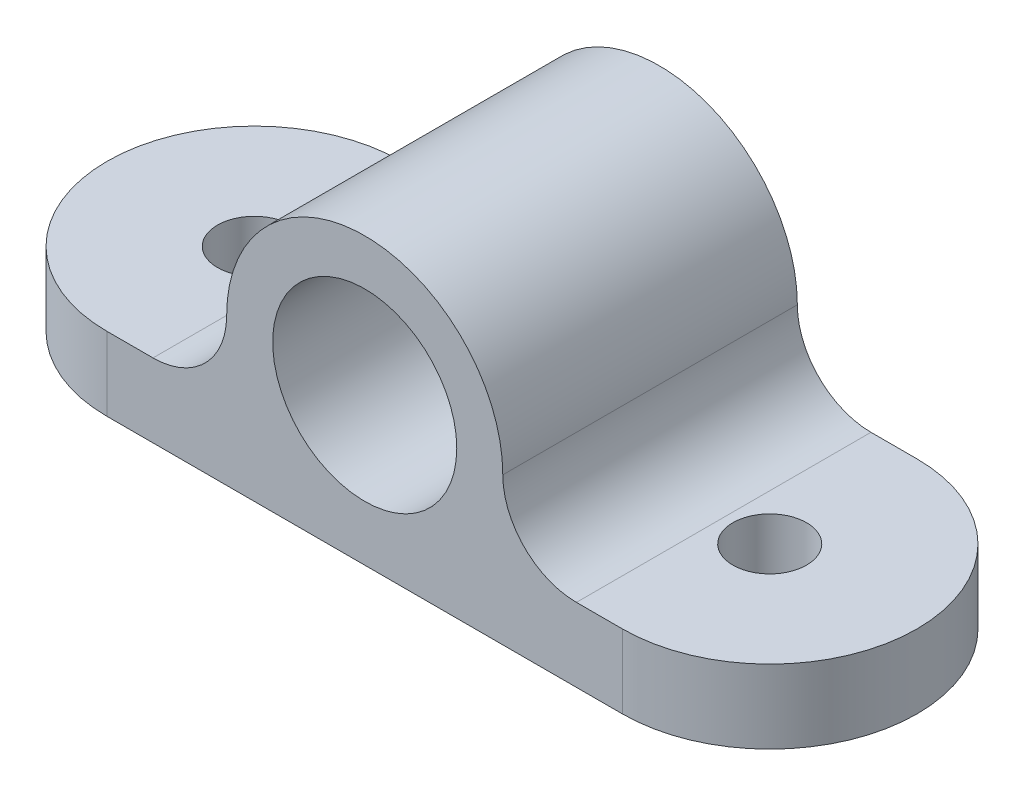
ISO-10303-21;
HEADER;
FILE_DESCRIPTION(('STEP AP214'),'2;1');
FILE_NAME('part.step','',(''),(''),'','','');
FILE_SCHEMA(('AUTOMOTIVE_DESIGN { 1 0 10303 214 1 1 1 1 }'));
ENDSEC;
DATA;
#1=APPLICATION_CONTEXT('core data for automotive mechanical design processes');
#2=APPLICATION_PROTOCOL_DEFINITION('international standard','automotive_design',2000,#1);
#3=PRODUCT_CONTEXT('',#1,'mechanical');
#4=PRODUCT('Part','Part','',(#3));
#5=PRODUCT_RELATED_PRODUCT_CATEGORY('part','',(#4));
#6=PRODUCT_DEFINITION_FORMATION('','',#4);
#7=PRODUCT_DEFINITION_CONTEXT('part definition',#1,'design');
#8=PRODUCT_DEFINITION('design','',#6,#7);
#9=PRODUCT_DEFINITION_SHAPE('','',#8);
#10=(LENGTH_UNIT() NAMED_UNIT(*) SI_UNIT(.MILLI.,.METRE.));
#11=(NAMED_UNIT(*) PLANE_ANGLE_UNIT() SI_UNIT($,.RADIAN.));
#12=(NAMED_UNIT(*) SI_UNIT($,.STERADIAN.) SOLID_ANGLE_UNIT());
#13=UNCERTAINTY_MEASURE_WITH_UNIT(LENGTH_MEASURE(1.E-05),#10,'distance_accuracy_value','');
#14=(GEOMETRIC_REPRESENTATION_CONTEXT(3) GLOBAL_UNCERTAINTY_ASSIGNED_CONTEXT((#13)) GLOBAL_UNIT_ASSIGNED_CONTEXT((#10,
#11,#12)) REPRESENTATION_CONTEXT('',''));
#15=CARTESIAN_POINT('',(0.,0.,0.));
#16=DIRECTION('',(0.,0.,1.));
#17=DIRECTION('',(1.,0.,0.));
#18=AXIS2_PLACEMENT_3D('',#15,#16,#17);
#19=CARTESIAN_POINT('',(-70.,0.,40.));
#20=DIRECTION('',(0.,-1.,0.));
#21=DIRECTION('',(0.,0.,-1.));
#22=AXIS2_PLACEMENT_3D('',#19,#20,#21);
#23=CYLINDRICAL_SURFACE('',#22,40.);
#24=DIRECTION('',(0.,-1.,0.));
#25=VECTOR('',#24,1.);
#26=CARTESIAN_POINT('',(-70.,40.,0.));
#27=LINE('',#26,#25);
#28=CARTESIAN_POINT('',(-70.,0.,0.));
#29=VERTEX_POINT('',#28);
#30=CARTESIAN_POINT('',(-70.,20.,0.));
#31=VERTEX_POINT('',#30);
#32=EDGE_CURVE('E154',#29,#31,#27,.F.);
#33=ORIENTED_EDGE('',*,*,#32,.F.);
#34=CARTESIAN_POINT('',(-70.,0.,40.));
#35=DIRECTION('',(0.,1.,0.));
#36=DIRECTION('',(0.,0.,1.));
#37=AXIS2_PLACEMENT_3D('',#34,#35,#36);
#38=CIRCLE('',#37,40.);
#39=CARTESIAN_POINT('',(-70.,0.,80.));
#40=VERTEX_POINT('',#39);
#41=EDGE_CURVE('E49',#40,#29,#38,.F.);
#42=ORIENTED_EDGE('',*,*,#41,.F.);
#43=DIRECTION('',(0.,1.,0.));
#44=VECTOR('',#43,1.);
#45=CARTESIAN_POINT('',(-70.,0.,80.));
#46=LINE('',#45,#44);
#47=CARTESIAN_POINT('',(-70.,20.,80.));
#48=VERTEX_POINT('',#47);
#49=EDGE_CURVE('E158',#48,#40,#46,.F.);
#50=ORIENTED_EDGE('',*,*,#49,.F.);
#51=CARTESIAN_POINT('',(-70.,20.,40.));
#52=DIRECTION('',(0.,-1.,0.));
#53=DIRECTION('',(0.,0.,-1.));
#54=AXIS2_PLACEMENT_3D('',#51,#52,#53);
#55=CIRCLE('',#54,40.);
#56=EDGE_CURVE('E11',#31,#48,#55,.F.);
#57=ORIENTED_EDGE('',*,*,#56,.F.);
#58=EDGE_LOOP('',(#33,#42,#50,#57));
#59=FACE_BOUND('',#58,.T.);
#60=ADVANCED_FACE('F41',(#59),#23,.T.);
#61=CARTESIAN_POINT('',(70.,0.,40.));
#62=DIRECTION('',(0.,1.,0.));
#63=DIRECTION('',(0.,0.,1.));
#64=AXIS2_PLACEMENT_3D('',#61,#62,#63);
#65=CYLINDRICAL_SURFACE('',#64,40.);
#66=DIRECTION('',(0.,-1.,0.));
#67=VECTOR('',#66,1.);
#68=CARTESIAN_POINT('',(70.,0.,80.));
#69=LINE('',#68,#67);
#70=CARTESIAN_POINT('',(70.,0.,80.));
#71=VERTEX_POINT('',#70);
#72=CARTESIAN_POINT('',(70.,20.,80.));
#73=VERTEX_POINT('',#72);
#74=EDGE_CURVE('E145',#71,#73,#69,.F.);
#75=ORIENTED_EDGE('',*,*,#74,.F.);
#76=CARTESIAN_POINT('',(70.,0.,40.));
#77=DIRECTION('',(0.,1.,0.));
#78=DIRECTION('',(0.,0.,1.));
#79=AXIS2_PLACEMENT_3D('',#76,#77,#78);
#80=CIRCLE('',#79,40.);
#81=CARTESIAN_POINT('',(70.,0.,0.));
#82=VERTEX_POINT('',#81);
#83=EDGE_CURVE('E147',#82,#71,#80,.F.);
#84=ORIENTED_EDGE('',*,*,#83,.F.);
#85=DIRECTION('',(0.,1.,0.));
#86=VECTOR('',#85,1.);
#87=CARTESIAN_POINT('',(70.,40.,0.));
#88=LINE('',#87,#86);
#89=CARTESIAN_POINT('',(70.,20.,0.));
#90=VERTEX_POINT('',#89);
#91=EDGE_CURVE('E150',#90,#82,#88,.F.);
#92=ORIENTED_EDGE('',*,*,#91,.F.);
#93=CARTESIAN_POINT('',(70.,20.,40.));
#94=DIRECTION('',(0.,-1.,0.));
#95=DIRECTION('',(0.,0.,-1.));
#96=AXIS2_PLACEMENT_3D('',#93,#94,#95);
#97=CIRCLE('',#96,40.);
#98=EDGE_CURVE('E153',#73,#90,#97,.F.);
#99=ORIENTED_EDGE('',*,*,#98,.F.);
#100=EDGE_LOOP('',(#75,#84,#92,#99));
#101=FACE_BOUND('',#100,.T.);
#102=ADVANCED_FACE('F213',(#101),#65,.T.);
#103=CARTESIAN_POINT('',(0.,40.,80.));
#104=DIRECTION('',(0.,0.,1.));
#105=DIRECTION('',(1.,0.,0.));
#106=AXIS2_PLACEMENT_3D('',#103,#104,#105);
#107=PLANE('',#106);
#108=DIRECTION('',(-1.,0.,0.));
#109=VECTOR('',#108,1.);
#110=CARTESIAN_POINT('',(-37.5,20.,80.));
#111=LINE('',#110,#109);
#112=CARTESIAN_POINT('',(-57.5,20.,80.));
#113=VERTEX_POINT('',#112);
#114=EDGE_CURVE('E116',#113,#48,#111,.T.);
#115=ORIENTED_EDGE('',*,*,#114,.T.);
#116=ORIENTED_EDGE('',*,*,#49,.T.);
#117=DIRECTION('',(1.,0.,0.));
#118=VECTOR('',#117,1.);
#119=CARTESIAN_POINT('',(-110.,0.,80.));
#120=LINE('',#119,#118);
#121=EDGE_CURVE('E167',#40,#71,#120,.T.);
#122=ORIENTED_EDGE('',*,*,#121,.T.);
#123=ORIENTED_EDGE('',*,*,#74,.T.);
#124=DIRECTION('',(-1.,0.,0.));
#125=VECTOR('',#124,1.);
#126=CARTESIAN_POINT('',(110.,20.,80.));
#127=LINE('',#126,#125);
#128=CARTESIAN_POINT('',(57.5,20.,80.));
#129=VERTEX_POINT('',#128);
#130=EDGE_CURVE('E178',#73,#129,#127,.T.);
#131=ORIENTED_EDGE('',*,*,#130,.T.);
#132=CARTESIAN_POINT('',(57.5,40.,80.));
#133=DIRECTION('',(0.,0.,1.));
#134=DIRECTION('',(1.,0.,0.));
#135=AXIS2_PLACEMENT_3D('',#132,#133,#134);
#136=CIRCLE('',#135,20.);
#137=CARTESIAN_POINT('',(37.5,40.,80.));
#138=VERTEX_POINT('',#137);
#139=EDGE_CURVE('E115',#129,#138,#136,.F.);
#140=ORIENTED_EDGE('',*,*,#139,.T.);
#141=CARTESIAN_POINT('',(0.,40.,80.));
#142=DIRECTION('',(0.,0.,1.));
#143=DIRECTION('',(1.,0.,0.));
#144=AXIS2_PLACEMENT_3D('',#141,#142,#143);
#145=CIRCLE('',#144,37.5);
#146=CARTESIAN_POINT('',(-37.5,40.,80.));
#147=VERTEX_POINT('',#146);
#148=EDGE_CURVE('E102',#138,#147,#145,.T.);
#149=ORIENTED_EDGE('',*,*,#148,.T.);
#150=CARTESIAN_POINT('',(-57.5,40.,80.));
#151=DIRECTION('',(0.,0.,1.));
#152=DIRECTION('',(1.,0.,0.));
#153=AXIS2_PLACEMENT_3D('',#150,#151,#152);
#154=CIRCLE('',#153,20.);
#155=EDGE_CURVE('E109',#147,#113,#154,.F.);
#156=ORIENTED_EDGE('',*,*,#155,.T.);
#157=EDGE_LOOP('',(#115,#116,#122,#123,#131,#140,#149,#156));
#158=FACE_BOUND('',#157,.T.);
#159=CARTESIAN_POINT('',(0.,40.,80.));
#160=DIRECTION('',(0.,0.,1.));
#161=DIRECTION('',(1.,0.,0.));
#162=AXIS2_PLACEMENT_3D('',#159,#160,#161);
#163=CIRCLE('',#162,25.);
#164=CARTESIAN_POINT('',(25.,40.,80.));
#165=VERTEX_POINT('',#164);
#166=EDGE_CURVE('E185',#165,#165,#163,.T.);
#167=ORIENTED_EDGE('',*,*,#166,.F.);
#168=EDGE_LOOP('',(#167));
#169=FACE_BOUND('',#168,.T.);
#170=ADVANCED_FACE('F110',(#158,#169),#107,.T.);
#171=CARTESIAN_POINT('',(0.,40.,0.));
#172=DIRECTION('',(0.,0.,1.));
#173=DIRECTION('',(1.,0.,0.));
#174=AXIS2_PLACEMENT_3D('',#171,#172,#173);
#175=PLANE('',#174);
#176=DIRECTION('',(1.,0.,0.));
#177=VECTOR('',#176,1.);
#178=CARTESIAN_POINT('',(-110.,0.,0.));
#179=LINE('',#178,#177);
#180=EDGE_CURVE('E163',#29,#82,#179,.T.);
#181=ORIENTED_EDGE('',*,*,#180,.F.);
#182=ORIENTED_EDGE('',*,*,#32,.T.);
#183=DIRECTION('',(-1.,0.,0.));
#184=VECTOR('',#183,1.);
#185=CARTESIAN_POINT('',(-110.,20.,0.));
#186=LINE('',#185,#184);
#187=CARTESIAN_POINT('',(-57.5,20.,0.));
#188=VERTEX_POINT('',#187);
#189=EDGE_CURVE('E174',#188,#31,#186,.T.);
#190=ORIENTED_EDGE('',*,*,#189,.F.);
#191=CARTESIAN_POINT('',(-57.5,40.,0.));
#192=DIRECTION('',(0.,0.,1.));
#193=DIRECTION('',(1.,0.,0.));
#194=AXIS2_PLACEMENT_3D('',#191,#192,#193);
#195=CIRCLE('',#194,20.);
#196=CARTESIAN_POINT('',(-37.5,40.,0.));
#197=VERTEX_POINT('',#196);
#198=EDGE_CURVE('E134',#188,#197,#195,.T.);
#199=ORIENTED_EDGE('',*,*,#198,.T.);
#200=CARTESIAN_POINT('',(0.,40.,0.));
#201=DIRECTION('',(0.,0.,1.));
#202=DIRECTION('',(1.,0.,0.));
#203=AXIS2_PLACEMENT_3D('',#200,#201,#202);
#204=CIRCLE('',#203,37.5);
#205=CARTESIAN_POINT('',(37.5,40.,0.));
#206=VERTEX_POINT('',#205);
#207=EDGE_CURVE('E123',#206,#197,#204,.T.);
#208=ORIENTED_EDGE('',*,*,#207,.F.);
#209=CARTESIAN_POINT('',(57.5,40.,0.));
#210=DIRECTION('',(0.,0.,1.));
#211=DIRECTION('',(1.,0.,0.));
#212=AXIS2_PLACEMENT_3D('',#209,#210,#211);
#213=CIRCLE('',#212,20.);
#214=CARTESIAN_POINT('',(57.5,20.,0.));
#215=VERTEX_POINT('',#214);
#216=EDGE_CURVE('E136',#206,#215,#213,.T.);
#217=ORIENTED_EDGE('',*,*,#216,.T.);
#218=DIRECTION('',(-1.,0.,0.));
#219=VECTOR('',#218,1.);
#220=CARTESIAN_POINT('',(37.5,20.,0.));
#221=LINE('',#220,#219);
#222=EDGE_CURVE('E117',#90,#215,#221,.T.);
#223=ORIENTED_EDGE('',*,*,#222,.F.);
#224=ORIENTED_EDGE('',*,*,#91,.T.);
#225=EDGE_LOOP('',(#181,#182,#190,#199,#208,#217,#223,#224));
#226=FACE_BOUND('',#225,.T.);
#227=CARTESIAN_POINT('',(0.,40.,0.));
#228=DIRECTION('',(0.,0.,1.));
#229=DIRECTION('',(1.,0.,0.));
#230=AXIS2_PLACEMENT_3D('',#227,#228,#229);
#231=CIRCLE('',#230,25.);
#232=CARTESIAN_POINT('',(25.,40.,0.));
#233=VERTEX_POINT('',#232);
#234=EDGE_CURVE('E184',#233,#233,#231,.T.);
#235=ORIENTED_EDGE('',*,*,#234,.T.);
#236=EDGE_LOOP('',(#235));
#237=FACE_BOUND('',#236,.T.);
#238=ADVANCED_FACE('F166',(#226,#237),#175,.F.);
#239=CARTESIAN_POINT('',(0.,40.,80.));
#240=DIRECTION('',(0.,0.,-1.));
#241=DIRECTION('',(-1.,0.,0.));
#242=AXIS2_PLACEMENT_3D('',#239,#240,#241);
#243=CYLINDRICAL_SURFACE('',#242,37.5);
#244=ORIENTED_EDGE('',*,*,#207,.T.);
#245=DIRECTION('',(0.,0.,-1.));
#246=VECTOR('',#245,1.);
#247=CARTESIAN_POINT('',(-37.5,40.,80.));
#248=LINE('',#247,#246);
#249=EDGE_CURVE('E121',#147,#197,#248,.T.);
#250=ORIENTED_EDGE('',*,*,#249,.F.);
#251=ORIENTED_EDGE('',*,*,#148,.F.);
#252=DIRECTION('',(0.,0.,-1.));
#253=VECTOR('',#252,1.);
#254=CARTESIAN_POINT('',(37.5,40.,80.));
#255=LINE('',#254,#253);
#256=EDGE_CURVE('E130',#138,#206,#255,.T.);
#257=ORIENTED_EDGE('',*,*,#256,.T.);
#258=EDGE_LOOP('',(#244,#250,#251,#257));
#259=FACE_BOUND('',#258,.T.);
#260=ADVANCED_FACE('F122',(#259),#243,.T.);
#261=CARTESIAN_POINT('',(-110.,20.,80.));
#262=DIRECTION('',(0.,-1.,0.));
#263=DIRECTION('',(0.,0.,-1.));
#264=AXIS2_PLACEMENT_3D('',#261,#262,#263);
#265=PLANE('',#264);
#266=CARTESIAN_POINT('',(-70.,20.,40.));
#267=DIRECTION('',(0.,1.,0.));
#268=DIRECTION('',(0.,0.,1.));
#269=AXIS2_PLACEMENT_3D('',#266,#267,#268);
#270=CIRCLE('',#269,10.);
#271=CARTESIAN_POINT('',(-70.,20.,50.));
#272=VERTEX_POINT('',#271);
#273=EDGE_CURVE('E198',#272,#272,#270,.T.);
#274=ORIENTED_EDGE('',*,*,#273,.F.);
#275=EDGE_LOOP('',(#274));
#276=FACE_BOUND('',#275,.T.);
#277=ORIENTED_EDGE('',*,*,#189,.T.);
#278=ORIENTED_EDGE('',*,*,#56,.T.);
#279=ORIENTED_EDGE('',*,*,#114,.F.);
#280=DIRECTION('',(0.,0.,-1.));
#281=VECTOR('',#280,1.);
#282=CARTESIAN_POINT('',(-57.5,20.,0.));
#283=LINE('',#282,#281);
#284=EDGE_CURVE('E127',#113,#188,#283,.T.);
#285=ORIENTED_EDGE('',*,*,#284,.T.);
#286=EDGE_LOOP('',(#277,#278,#279,#285));
#287=FACE_BOUND('',#286,.T.);
#288=ADVANCED_FACE('F180',(#276,#287),#265,.F.);
#289=CARTESIAN_POINT('',(-110.,0.,80.));
#290=DIRECTION('',(0.,1.,0.));
#291=DIRECTION('',(0.,0.,1.));
#292=AXIS2_PLACEMENT_3D('',#289,#290,#291);
#293=PLANE('',#292);
#294=CARTESIAN_POINT('',(70.,0.,40.));
#295=DIRECTION('',(0.,1.,0.));
#296=DIRECTION('',(0.,0.,1.));
#297=AXIS2_PLACEMENT_3D('',#294,#295,#296);
#298=CIRCLE('',#297,9.99999999999999);
#299=CARTESIAN_POINT('',(70.,0.,50.));
#300=VERTEX_POINT('',#299);
#301=EDGE_CURVE('E192',#300,#300,#298,.T.);
#302=ORIENTED_EDGE('',*,*,#301,.T.);
#303=EDGE_LOOP('',(#302));
#304=FACE_BOUND('',#303,.T.);
#305=CARTESIAN_POINT('',(-70.,0.,40.));
#306=DIRECTION('',(0.,1.,0.));
#307=DIRECTION('',(0.,0.,1.));
#308=AXIS2_PLACEMENT_3D('',#305,#306,#307);
#309=CIRCLE('',#308,10.);
#310=CARTESIAN_POINT('',(-70.,0.,50.));
#311=VERTEX_POINT('',#310);
#312=EDGE_CURVE('E44',#311,#311,#309,.T.);
#313=ORIENTED_EDGE('',*,*,#312,.T.);
#314=EDGE_LOOP('',(#313));
#315=FACE_BOUND('',#314,.T.);
#316=ORIENTED_EDGE('',*,*,#121,.F.);
#317=ORIENTED_EDGE('',*,*,#41,.T.);
#318=ORIENTED_EDGE('',*,*,#180,.T.);
#319=ORIENTED_EDGE('',*,*,#83,.T.);
#320=EDGE_LOOP('',(#316,#317,#318,#319));
#321=FACE_BOUND('',#320,.T.);
#322=ADVANCED_FACE('F165',(#304,#315,#321),#293,.F.);
#323=CARTESIAN_POINT('',(37.5,20.,80.));
#324=DIRECTION('',(0.,-1.,0.));
#325=DIRECTION('',(0.,0.,-1.));
#326=AXIS2_PLACEMENT_3D('',#323,#324,#325);
#327=PLANE('',#326);
#328=CARTESIAN_POINT('',(70.,20.,40.));
#329=DIRECTION('',(0.,1.,0.));
#330=DIRECTION('',(0.,0.,1.));
#331=AXIS2_PLACEMENT_3D('',#328,#329,#330);
#332=CIRCLE('',#331,9.99999999999999);
#333=CARTESIAN_POINT('',(70.,20.,50.));
#334=VERTEX_POINT('',#333);
#335=EDGE_CURVE('E195',#334,#334,#332,.T.);
#336=ORIENTED_EDGE('',*,*,#335,.F.);
#337=EDGE_LOOP('',(#336));
#338=FACE_BOUND('',#337,.T.);
#339=ORIENTED_EDGE('',*,*,#130,.F.);
#340=ORIENTED_EDGE('',*,*,#98,.T.);
#341=ORIENTED_EDGE('',*,*,#222,.T.);
#342=DIRECTION('',(0.,0.,-1.));
#343=VECTOR('',#342,1.);
#344=CARTESIAN_POINT('',(57.5,20.,80.));
#345=LINE('',#344,#343);
#346=EDGE_CURVE('E132',#215,#129,#345,.F.);
#347=ORIENTED_EDGE('',*,*,#346,.T.);
#348=EDGE_LOOP('',(#339,#340,#341,#347));
#349=FACE_BOUND('',#348,.T.);
#350=ADVANCED_FACE('F202',(#338,#349),#327,.F.);
#351=CARTESIAN_POINT('',(0.,40.,80.));
#352=DIRECTION('',(0.,0.,-1.));
#353=DIRECTION('',(-1.,0.,0.));
#354=AXIS2_PLACEMENT_3D('',#351,#352,#353);
#355=CYLINDRICAL_SURFACE('',#354,25.);
#356=ORIENTED_EDGE('',*,*,#166,.T.);
#357=EDGE_LOOP('',(#356));
#358=FACE_BOUND('',#357,.T.);
#359=ORIENTED_EDGE('',*,*,#234,.F.);
#360=EDGE_LOOP('',(#359));
#361=FACE_BOUND('',#360,.T.);
#362=ADVANCED_FACE('F208',(#358,#361),#355,.F.);
#363=CARTESIAN_POINT('',(-57.5,40.,80.));
#364=DIRECTION('',(0.,0.,1.));
#365=DIRECTION('',(1.,0.,0.));
#366=AXIS2_PLACEMENT_3D('',#363,#364,#365);
#367=CYLINDRICAL_SURFACE('',#366,20.);
#368=ORIENTED_EDGE('',*,*,#155,.F.);
#369=ORIENTED_EDGE('',*,*,#249,.T.);
#370=ORIENTED_EDGE('',*,*,#198,.F.);
#371=ORIENTED_EDGE('',*,*,#284,.F.);
#372=EDGE_LOOP('',(#368,#369,#370,#371));
#373=FACE_BOUND('',#372,.T.);
#374=ADVANCED_FACE('F128',(#373),#367,.F.);
#375=CARTESIAN_POINT('',(57.5,40.,80.));
#376=DIRECTION('',(0.,0.,1.));
#377=DIRECTION('',(1.,0.,0.));
#378=AXIS2_PLACEMENT_3D('',#375,#376,#377);
#379=CYLINDRICAL_SURFACE('',#378,20.);
#380=ORIENTED_EDGE('',*,*,#139,.F.);
#381=ORIENTED_EDGE('',*,*,#346,.F.);
#382=ORIENTED_EDGE('',*,*,#216,.F.);
#383=ORIENTED_EDGE('',*,*,#256,.F.);
#384=EDGE_LOOP('',(#380,#381,#382,#383));
#385=FACE_BOUND('',#384,.T.);
#386=ADVANCED_FACE('F223',(#385),#379,.F.);
#387=CARTESIAN_POINT('',(70.,-60.,40.));
#388=DIRECTION('',(0.,1.,0.));
#389=DIRECTION('',(0.,0.,1.));
#390=AXIS2_PLACEMENT_3D('',#387,#388,#389);
#391=CYLINDRICAL_SURFACE('',#390,9.99999999999999);
#392=ORIENTED_EDGE('',*,*,#335,.T.);
#393=EDGE_LOOP('',(#392));
#394=FACE_BOUND('',#393,.T.);
#395=ORIENTED_EDGE('',*,*,#301,.F.);
#396=EDGE_LOOP('',(#395));
#397=FACE_BOUND('',#396,.T.);
#398=ADVANCED_FACE('F205',(#394,#397),#391,.F.);
#399=CARTESIAN_POINT('',(-70.,-60.,40.));
#400=DIRECTION('',(0.,1.,0.));
#401=DIRECTION('',(0.,0.,1.));
#402=AXIS2_PLACEMENT_3D('',#399,#400,#401);
#403=CYLINDRICAL_SURFACE('',#402,10.);
#404=ORIENTED_EDGE('',*,*,#273,.T.);
#405=EDGE_LOOP('',(#404));
#406=FACE_BOUND('',#405,.T.);
#407=ORIENTED_EDGE('',*,*,#312,.F.);
#408=EDGE_LOOP('',(#407));
#409=FACE_BOUND('',#408,.T.);
#410=ADVANCED_FACE('F244',(#406,#409),#403,.F.);
#411=CLOSED_SHELL('',(#60,#102,#170,#238,#260,#288,#322,#350,#362,#374,#386,#398,#410));
#412=MANIFOLD_SOLID_BREP('B2',#411);
#413=ADVANCED_BREP_SHAPE_REPRESENTATION('',(#18,#412),#14);
#414=SHAPE_DEFINITION_REPRESENTATION(#9,#413);
ENDSEC;
END-ISO-10303-21;
